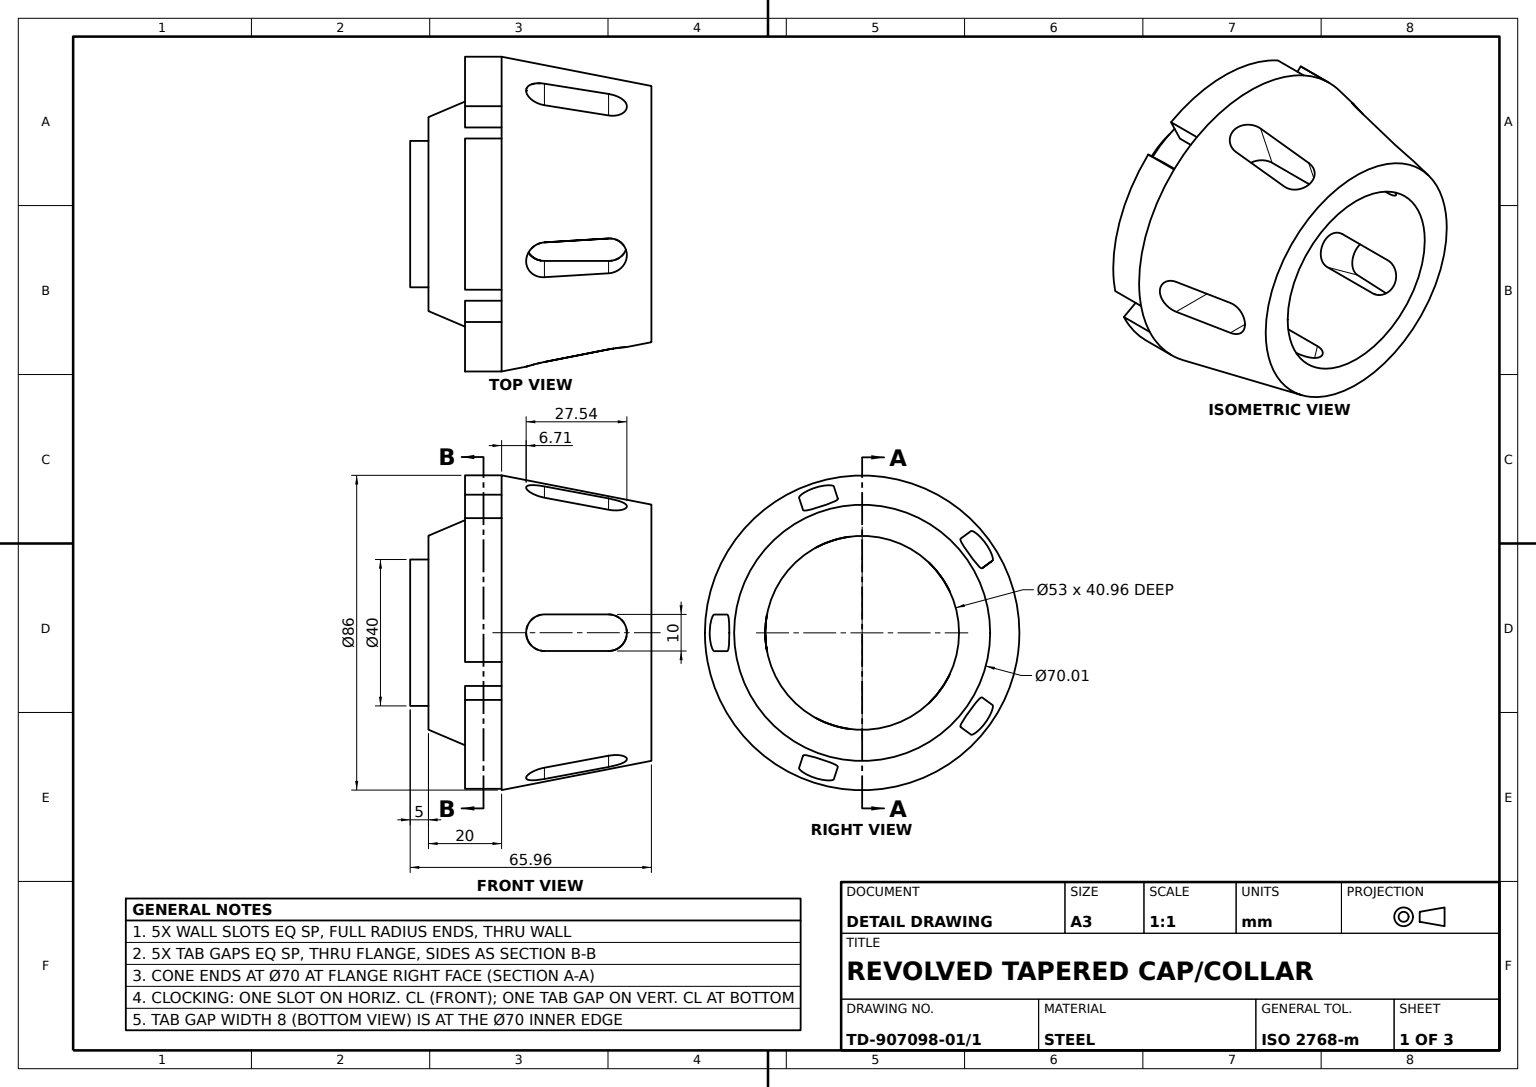
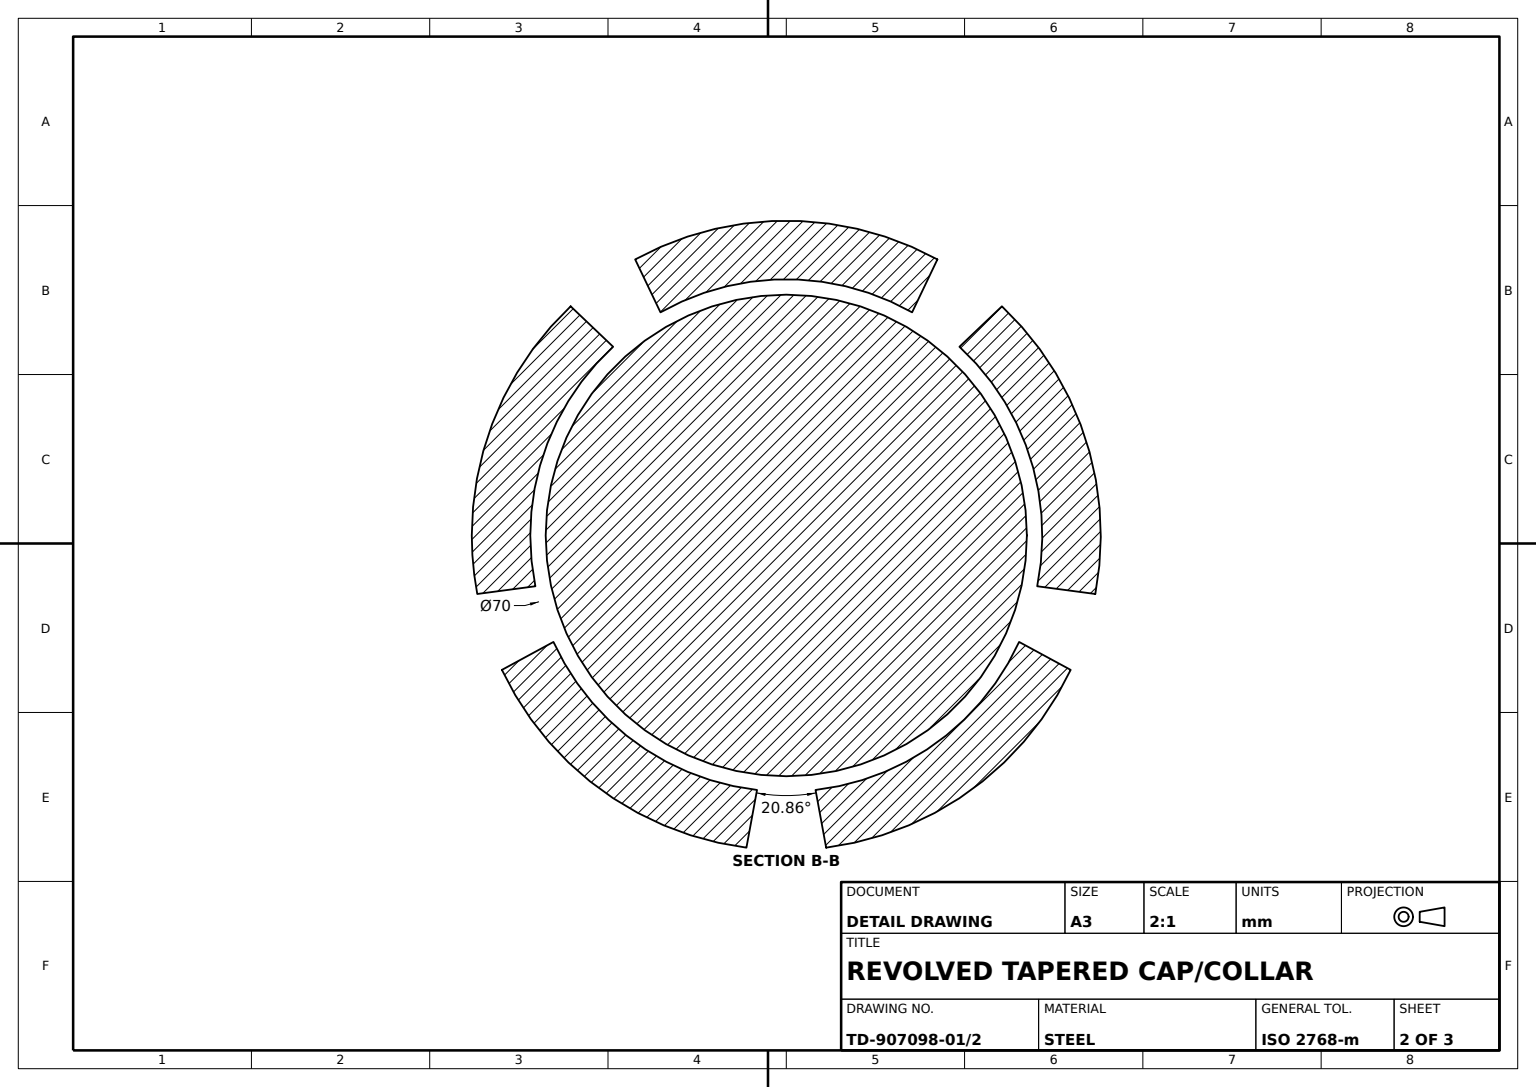
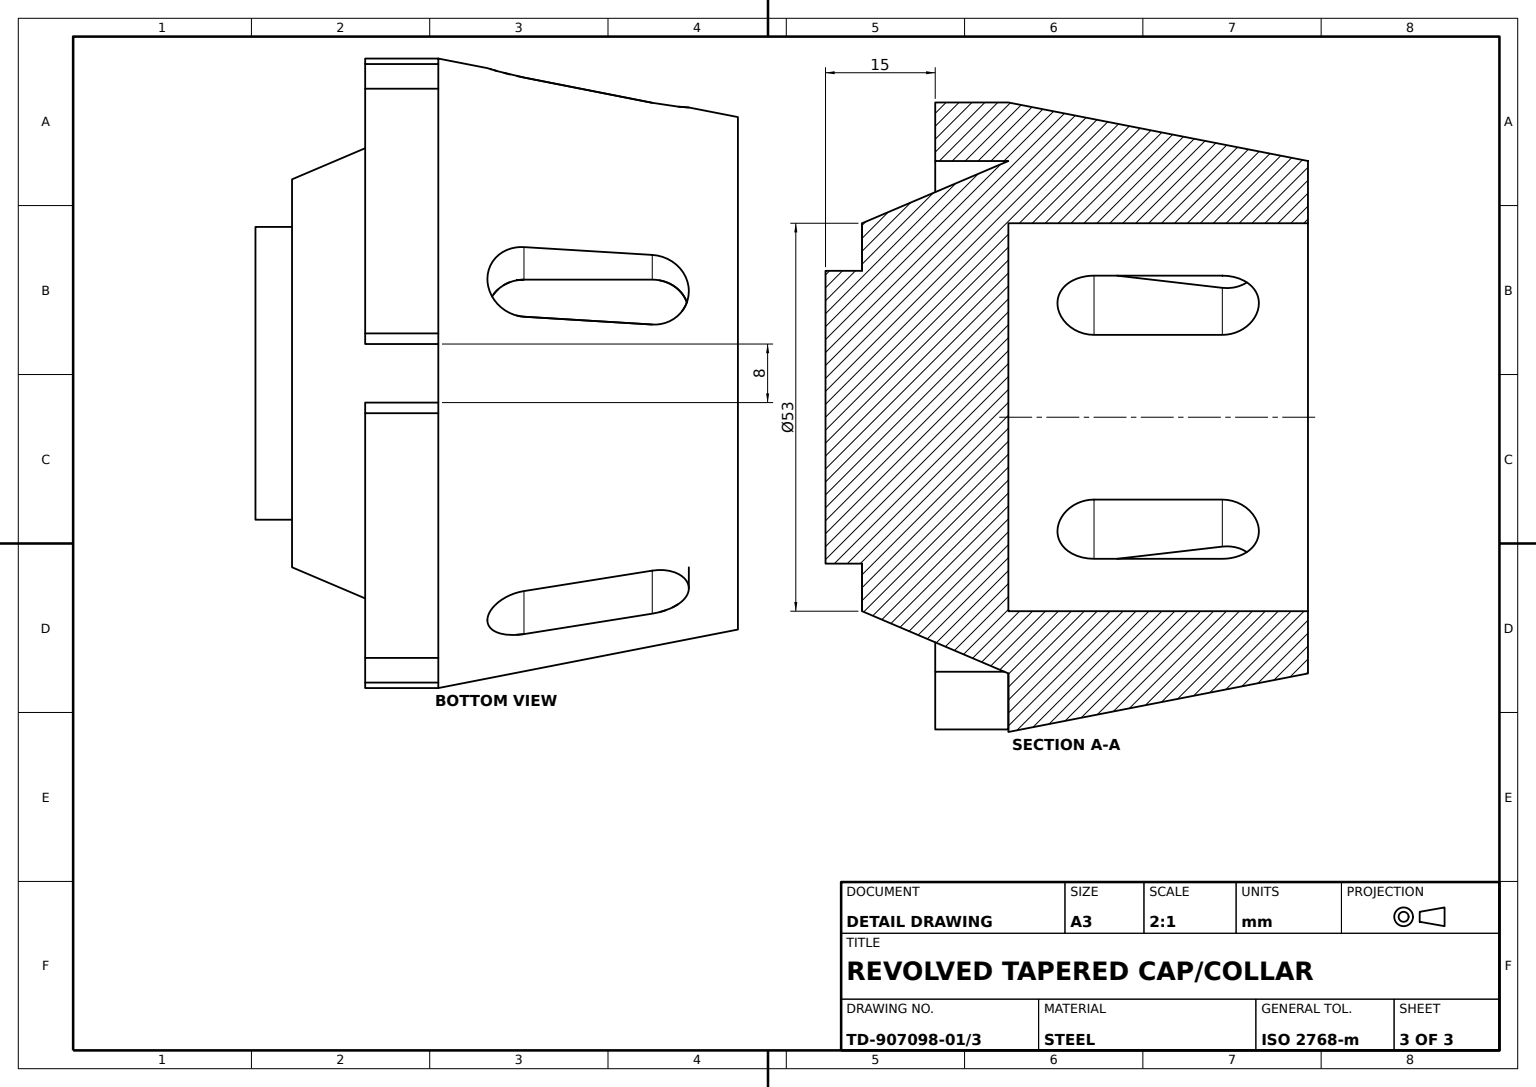
from build123d import *

# Parameters (mm, degrees)
WALL_SLOT_CUT_REACH        = 91.715
WALL_SLOT_PATTERN_5X_COUNT = 5
BASE_TABS_DEPTH            = 10


with BuildPart() as part:
    # Housing Profile Sketch → Tapered Housing Body (revolve)
    with BuildSketch(Plane.XY, mode=Mode.PRIVATE) as tapered_housing_body_sk:
        Polygon((0, 0), (-20, 0), (-20, 5), (-26.5, 5), (-35, 25), (-43, 25), (-35.005, 65.96), (-26.5, 65.96), (-26.5, 25), (0, 25), align=None)
    revolve(tapered_housing_body_sk.sketch.rotate(Axis((0, 0, 0), (0, 1, 0)), 270), axis=Axis((0, 0, 0), (0, 1, 0)))

    # Wall Slot Cut: up to this cone (the profile starts inside it)
    wall_slot_cut_end = Plane(origin=(0, 45.48, 0), z_dir=(0, -1, 0)) * Cone(13.390099792, 64.614900208, 262.435, mode=Mode.PRIVATE)
    # Wall Slot Sketch → Wall Slot Cut (cut, up to the surface)
    with BuildSketch(Plane.XY, mode=Mode.PRIVATE) as wall_slot_cut_sk1:
        with BuildLine():
            Line((5, 54.25), (5, 36.71))
            ThreePointArc((5, 36.71), (0, 31.71), (-5, 36.71))
            Line((-5, 36.71), (-5, 54.25))
            ThreePointArc((-5, 54.25), (0, 59.25), (5, 54.25))
        make_face()
    wall_slot_cut_tool1 = extrude(wall_slot_cut_sk1.sketch, amount=WALL_SLOT_CUT_REACH, mode=Mode.PRIVATE) & wall_slot_cut_end
    wall_slot_cut = wall_slot_cut_tool1.solids().sort_by_distance((0, 45.48, 0))[0]
    add(wall_slot_cut, mode=Mode.SUBTRACT)

    # Wall Slot Pattern 5x: Wall Slot Cut ×5 about axis
    wall_slot_pattern_5x_axis = Axis((0, 0, 0), (0, 1, 0))
    for i in range(1, WALL_SLOT_PATTERN_5X_COUNT):
        add(wall_slot_cut.rotate(wall_slot_pattern_5x_axis, i * 360 / WALL_SLOT_PATTERN_5X_COUNT), mode=Mode.SUBTRACT)

    # Base Tab Sketch → Base Tabs (add)
    with BuildSketch(Plane.XZ.offset(-25)):
        with BuildLine():
            Line((34.770677301, 4), (42.65310085, 5.450962103))
            ThreePointArc((42.65310085, 5.450962103), (34.787730758, 25.274765849), (18.364706053, 38.881069579))
            Line((18.364706053, 38.881069579), (14.548956257, 31.832811246))
            ThreePointArc((14.548956257, 31.832811246), (28.315594803, 20.57248383), (34.770677301, 4))
        make_face()
        with BuildLine():
            Line((34.770677301, -4), (42.65310085, -5.450962103))
            ThreePointArc((42.65310085, -5.450962103), (34.787730758, -25.274765849), (18.364706053, -38.881069579))
            Line((18.364706053, -38.881069579), (14.548956257, -31.832811246))
            ThreePointArc((14.548956257, -31.832811246), (28.315594803, -20.57248383), (34.770677301, -4))
        make_face()
        with BuildLine():
            Line((6.940504127, -34.304947201), (7.996359998, -42.249949429))
            ThreePointArc((7.996359998, -42.249949429), (-13.287730758, -40.895430201), (-31.303088316, -29.480784621))
            Line((-31.303088316, -29.480784621), (-25.778927834, -23.673759307))
            ThreePointArc((-25.778927834, -23.673759307), (-10.815594803, -33.28697807), (6.940504127, -34.304947201))
        make_face()
        with BuildLine():
            Line((-30.481209852, -17.201623352), (-37.711078585, -20.660942668))
            ThreePointArc((-37.711078585, -20.660942668), (-43, 0), (-37.711078585, 20.660942668))
            Line((-37.711078585, 20.660942668), (-30.481209852, 17.201623353))
            ThreePointArc((-30.481209852, 17.201623353), (-35, 0), (-30.481209852, -17.201623352))
        make_face()
        with BuildLine():
            Line((-25.778927834, 23.673759307), (-31.303088316, 29.480784621))
            ThreePointArc((-31.303088316, 29.480784621), (-13.287730758, 40.895430201), (7.996359998, 42.249949429))
            Line((7.996359998, 42.249949429), (6.940504127, 34.304947201))
            ThreePointArc((6.940504127, 34.304947201), (-10.815594803, 33.28697807), (-25.778927834, 23.673759307))
        make_face()
    extrude(amount=BASE_TABS_DEPTH)


solid = part.part
